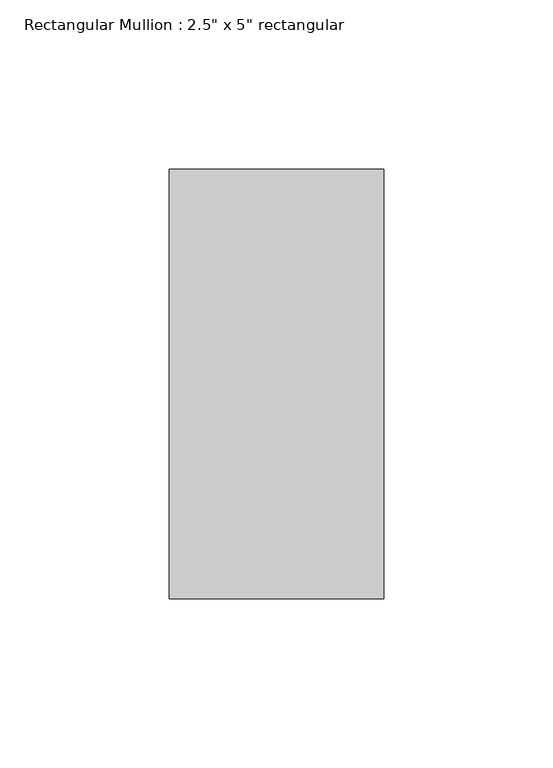
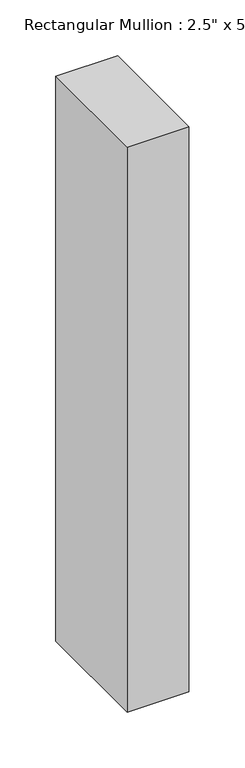
"""IFC4 building model written with IfcOpenShell, lengths in millimetres: member geometry."""

from ifc_helpers import new_model, si_unit, frame, origin, place, context, project, spatial, polyline, outline, extrude, source, transform, mapped, element, save


def member_f8dc38bf(model_context):
    return source(origin(), model_context, "Body", "SweptSolid", [
        extrude(outline(polyline([(31.75, 63.5), (31.75, -63.5), (-31.75, -63.5), (-31.75, 63.5), (31.75, 63.5)])), frame((0.0, 0.0, -615.95), z_axis=(0.0, 0.0, 1.0), x_axis=(1.0, 0.0, 0.0)), (0.0, 0.0, 1.0), 615.95),
    ])


if __name__ == "__main__":
    model = new_model("IFC4")
    model_context = context("Model", 3, world=origin())
    ifc_project = project(units=[si_unit("LENGTHUNIT", "METRE", prefix="MILLI")], contexts=[model_context])
    site = spatial("IfcSite", under=ifc_project)
    building = spatial("IfcBuilding", under=site)
    placement = place(None, origin())
    member_shape = member_f8dc38bf(model_context)
    element("IfcMember", 1, ObjectType="Rectangular Mullion : 2.5\" x 5\" rectangular", at=placement, inside=building, context=model_context, shape_type="MappedRepresentation", body=[
        mapped(member_shape, transform((0.0, 0.0, 0.0), x_axis=(1.0, 0.0, 0.0), y_axis=(0.0, 1.0, 0.0), z_axis=(0.0, 0.0, 1.0))),
    ])
    save(model, "model.ifc")

# Revit data of these elements
# Type "Rectangular Mullion : 2.5\" x 5\" rectangular"
#   built-in parameter 1007304 = 0.416667 (stored number, unit not read)
#   built-in parameter 1007301 = 0.104167 (stored number, unit not read)
#   built-in parameter 1007300 = 0.104167 (stored number, unit not read)
# Element 1 (IfcMember, "Rectangular Mullion : 2.5\" x 5\" rectangular")
#   Materials on its faces: "Aluminum"
# Materials
#   "Aluminum": class "Metal", colour RGB 247 247 247, transparency 0, Description = "Aluminum 6061", Cost = 0
